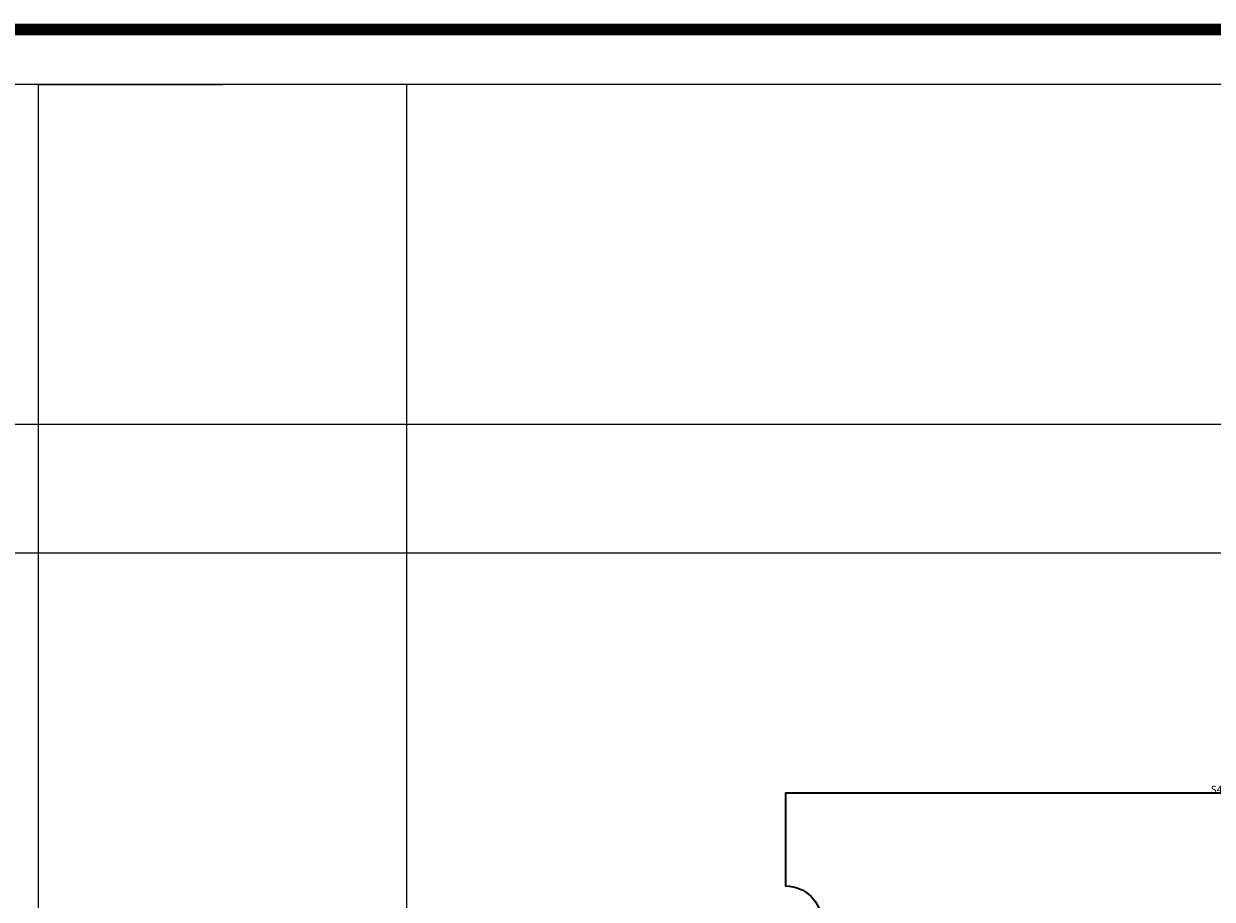
# Model space of a CAD drawing. Units: millimetres. Extents: x 353872 to 441597, y 126154 to 187356.
# Tile 25 of 28: x 399262 to 415084, y 175703 to 187356. Entities that reach past the tile are written whole.
import ezdxf

# ---------------------------------------------------------------- set-up
doc = ezdxf.new("R2010")
doc.units = ezdxf.units.MM
for name, color, linetype, lineweight in [('A-ANNO-DIMS', 2, 'Continuous', 18), ('P-ANNO-TEXT', 7, 'Continuous', 25), ('P-ANNO-TTLB', 7, 'Continuous', 25), ('P-PIPE', 3, 'Continuous', 35)]:
    doc.layers.add(name, color=color, linetype=linetype, lineweight=lineweight)
doc.styles.get("Standard").update_dxf_attribs({"font": 'arial.ttf'})
doc.dimstyles.get("Standard").update_dxf_attribs({"dimtxt": 0.18, "dimasz": 0.18, "dimexe": 0.18, "dimexo": 0.0625, "dimgap": 0.09, "dimtad": 0, "dimtih": 1, "dimtoh": 1, "dimdec": 4, "dimzin": 0, "dimdsep": 46, "dimtxsty": 'Standard', "dimcen": 0.09, "dimadec": 0, "dimazin": 0, "dimtfac": 1, "dimtdec": 4, "dimtofl": 0, "dimtmove": 0, "dimatfit": 3, "dimfxl": 1, "dimtolj": 1, "dimtzin": 0, "dimarcsym": 0})

# ---------------------------------------------------------------- blocks, each defined once
blk = doc.blocks.new('*D24')
at = {"layer": 'A-ANNO-DIMS', "color": 0, "lineweight": -2, "transparency": 16777216}
for p, q in [((360736.5468020001, 182546.115474), (360736.5468020001, 186546.232974)), ((360736.7268020001, 186546.052974), (396698.3316354127, 186546.052974)), ((432660.791653, 186546.052974), (396699.1868195874, 186546.052974)), ((432660.971653, 177114.47701), (432660.971653, 186546.232974))]:
    blk.add_line(p, q, dxfattribs=at)
at = {"layer": 'A-ANNO-DIMS', "color": 0, "transparency": 16777216}
for points in [[(360736.7268020001, 186546.082974), (360736.7268020001, 186546.022974), (360736.5468020001, 186546.052974)], [(432660.791653, 186546.082974), (432660.791653, 186546.022974), (432660.971653, 186546.052974)]]:
    blk.add_solid(points, dxfattribs=at)
at = {"layer": 'Defpoints', "color": 0, "transparency": 16777216}
for p in [(432660.971653, 186546.052974), (360736.5468020001, 182546.052974), (432660.971653, 177114.41451)]:
    blk.add_point(p, dxfattribs=at)
at = {"layer": 'A-ANNO-DIMS', "color": 0, "transparency": 16777216, "insert": (396698.7592275, 186546.052974), "char_height": 0.18, "attachment_point": 5}
blk.add_mtext('\\A1;71924', dxfattribs=at)
blk = doc.blocks.new('*D28')
at = {"layer": 'A-ANNO-DIMS', "color": 0, "lineweight": -2, "transparency": 16777216}
for p, q in [((366976.8176870001, 182028.441206), (440591.1818100004, 182028.441206)), ((440591.0018100004, 182028.261206), (440591.0018100004, 181171.3594706378)), ((440591.0018100004, 180314.093929), (440591.0018100004, 181170.9956643622)), ((366976.8176870001, 180313.913929), (440591.1818100004, 180313.913929))]:
    blk.add_line(p, q, dxfattribs=at)
at = {"layer": 'A-ANNO-DIMS', "color": 0, "transparency": 16777216}
for points in [[(440590.9718100004, 182028.261206), (440591.0318100004, 182028.261206), (440591.0018100004, 182028.441206)], [(440590.9718100004, 180314.093929), (440591.0318100004, 180314.093929), (440591.0018100004, 180313.913929)]]:
    blk.add_solid(points, dxfattribs=at)
at = {"layer": 'Defpoints', "color": 0, "transparency": 16777216}
for p in [(366976.7551870001, 182028.441206), (366976.7551870001, 180313.913929), (440591.0018100004, 180313.913929)]:
    blk.add_point(p, dxfattribs=at)
at = {"layer": 'A-ANNO-DIMS', "color": 0, "transparency": 16777216, "insert": (440591.0018100004, 181171.1775674999), "char_height": 0.18, "attachment_point": 5}
blk.add_mtext('\\A1;1714.5', dxfattribs=at)
blk = doc.blocks.new('*D33')
at = {"layer": 'A-ANNO-DIMS', "color": 0, "lineweight": -2, "transparency": 16777216}
for p, q in [((399457.1528810001, 167930.029452), (399457.1528810001, 186546.232974)), ((399457.332881, 186546.052974), (401909.7974381215, 186546.052974)), ((404362.9866609999, 186546.052974), (401910.5221038786, 186546.052974)), ((404363.1666609999, 167930.029452), (404363.1666609999, 186546.232974))]:
    blk.add_line(p, q, dxfattribs=at)
at = {"layer": 'A-ANNO-DIMS', "color": 0, "transparency": 16777216}
for points in [[(399457.332881, 186546.082974), (399457.332881, 186546.022974), (399457.1528810001, 186546.052974)], [(404362.9866609999, 186546.082974), (404362.9866609999, 186546.022974), (404363.1666609999, 186546.052974)]]:
    blk.add_solid(points, dxfattribs=at)
at = {"layer": 'Defpoints', "color": 0, "transparency": 16777216}
for p in [(404363.1666609999, 186546.052974), (399457.1528810001, 167929.966952), (404363.1666609999, 167929.966952)]:
    blk.add_point(p, dxfattribs=at)
at = {"layer": 'A-ANNO-DIMS', "color": 0, "transparency": 16777216, "insert": (401910.159771, 186546.052974), "char_height": 0.18, "attachment_point": 5}
blk.add_mtext('\\A1;4906', dxfattribs=at)

msp = doc.modelspace()

# ---------------------------------------------------------------- linework, layer by layer
at = {"layer": 'P-ANNO-TTLB', "const_width": 152.4336180244531}
msp.add_lwpolyline([(353948.027365095, 187280.0528919451), (353948.027365095, 126916.340154238), (440835.1896390488, 126916.340154238), (440835.1896390488, 187280.0528919451)], close=True, dxfattribs=at)
at = {"layer": 'P-PIPE'}
msp.add_lwpolyline([(426420.7632681744, 177114.4145097916), (409404.2253363539, 177114.4145097916), (409404.2253363539, 175879.9416156162, -0.9999999999999998), (409404.2253363539, 174919.8328494657), (409404.2253363542, 174162.7949221422, -0.9999999999997724), (409404.2253363539, 173202.6861559918), (409404.2253363539, 172914.6616783218), (409404.2253363539, 172512.0453955814)], format="xyb", dxfattribs=at)

# ---------------------------------------------------------------- texts
at = {"layer": 'P-ANNO-TEXT'}
msp.add_text('S4/50', height=98.09008979395831, dxfattribs=at).set_placement((415064.3458490805, 177114.4145097916))

# ---------------------------------------------------------------- dimensions: what is measured, and where the dimension line sits
at = {"layer": 'A-ANNO-DIMS'}
for base, p1, p2, picture, middle in [((432660.971653, 186546.052974), (360736.5468020001, 182546.052974), (432660.971653, 177114.41451), '*D24', (396698.7592275, 186546.052974)), ((404363.1666609999, 186546.052974), (399457.1528810001, 167929.966952), (404363.1666609999, 167929.966952), '*D33', (401910.159771, 186546.052974))]:
    dim = msp.add_linear_dim(base=base, p1=p1, p2=p2, dimstyle='Standard', override={"dimdec": 0, "dimlfac": 1, "dimrnd": 0, "dimzin": 0, "dimdsep": 46, "dimlunit": 2}, dxfattribs=at)
    dim.commit()
    dim.dimension.update_dxf_attribs({"geometry": picture, "text_midpoint": middle})
dim = msp.add_linear_dim(base=(440591.0018100004, 180313.913929), p1=(366976.7551870001, 182028.441206), p2=(366976.7551870001, 180313.913929), angle=90, dimstyle='Standard', override={"dimdec": 1, "dimlfac": 1, "dimrnd": 0, "dimzin": 0, "dimdsep": 46, "dimlunit": 2}, dxfattribs=at)
dim.commit()
dim.dimension.update_dxf_attribs({"geometry": '*D28', "text_midpoint": (440591.0018100004, 181171.1775674999)})

doc.saveas('drawing.dxf')
